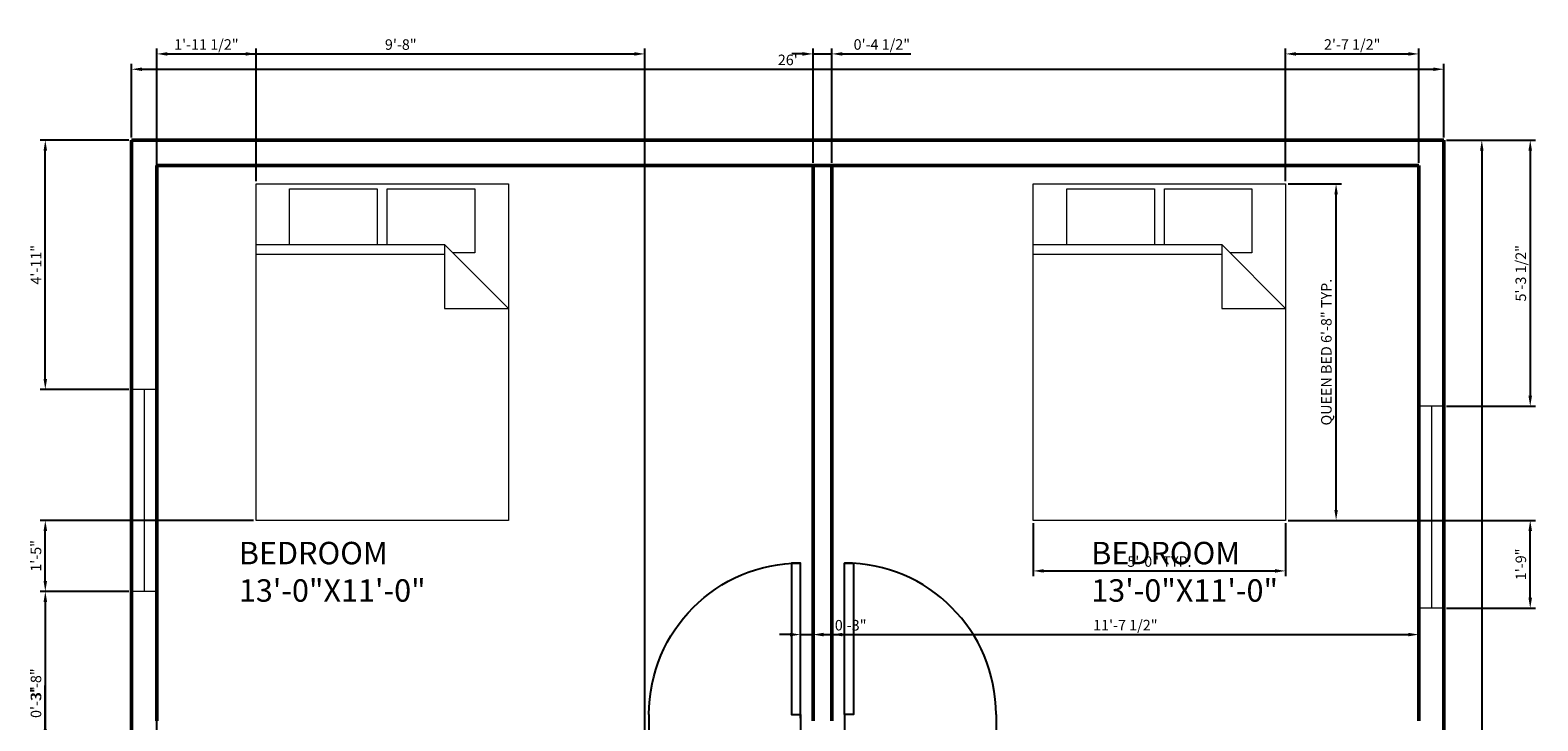
# Model space of a CAD drawing. Units: inches. Extents: x 158445 to 158806, y 254100 to 254533.
# Tile 3 of 3: x 158447 to 158806, y 254369 to 254533. Entities that reach past the tile are written whole.
import ezdxf

# ---------------------------------------------------------------- set-up
doc = ezdxf.new("R2010")
doc.units = ezdxf.units.IN
for name, color, linetype, lineweight in [('A-ANNO-DIMS', 2, 'Continuous', 18), ('A-AREA-IDEN', 7, 'Continuous', 25), ('A-DOOR', 3, 'Continuous', 25), ('A-FURN', 8, 'Continuous', 18), ('A-GLAZ', 4, 'Continuous', 18), ('A-WALL', 7, 'Continuous', 50)]:
    doc.layers.add(name, color=color, linetype=linetype, lineweight=lineweight)
doc.styles.get("Standard").update_dxf_attribs({"font": 'arial.ttf'})
doc.dimstyles.new('ISO-25', dxfattribs={"dimtxt": 2.5, "dimasz": 2.5, "dimexe": 1.25, "dimexo": 0.625, "dimtad": 1, "dimlunit": 4, "dimtxsty": 'Standard', "dimcen": 2.5, "dimadec": 0, "dimazin": 0, "dimtfac": 1, "dimtmove": 0, "dimatfit": 3, "dimfxl": 1, "dimarcsym": 0})

# ---------------------------------------------------------------- blocks, each defined once
blk = doc.blocks.new('*U2')
for p, q in [((0, 0), (0, -5)), ((30, 0), (30, -5))]:
    blk.add_line(p, q)
blk.add_lwpolyline([(0, 0), (0, 30), (1.75, 30), (1.75, 0)], close=True)
blk.add_arc((0, 0), 30, 0, 90)
blk = doc.blocks.new('Bed - Queen')
for p, q in [((0, -80.00003), (0, 0)), ((0, 0), (59.99999, 0)), ((59.99999, 0), (59.99999, -80.00003)), ((7.99999, -1.2), (28.79998, -1.2)), ((7.99999, -14.4), (7.99999, -1.2)), ((28.79998, -1.2), (28.79998, -14.4)), ((31.19999, -1.2), (51.99999, -1.2)), ((31.19999, -14.4), (31.19999, -1.2)), ((51.99999, -1.2), (51.99999, -16.4)), ((0, -14.4), (44.8, -14.4)), ((44.8, -16.8), (0, -16.8)), ((59.99999, -29.6), (44.8, -14.4)), ((44.8, -14.4), (44.8, -29.6)), ((51.99999, -16.4), (46.79936, -16.4)), ((44.8, -29.6), (59.99999, -29.6)), ((59.99999, -80.00003), (0, -80.00003))]:
    blk.add_line(p, q)
blk = doc.blocks.new('*D6')
at = {"layer": 'A-ANNO-DIMS', "color": 0, "lineweight": -2, "transparency": 16777216}
for p, q in [((158471.38, 254507.35), (158471.38, 254524.83)), ((158473.88, 254523.58), (158780.88, 254523.58)), ((158783.38, 254507.35), (158783.38, 254524.83))]:
    blk.add_line(p, q, dxfattribs=at)
at = {"layer": 'A-ANNO-DIMS', "color": 0, "transparency": 16777216}
for points in [[(158473.88, 254523.99), (158473.88, 254523.16), (158471.38, 254523.58)], [(158780.88, 254523.99), (158780.88, 254523.16), (158783.38, 254523.58)]]:
    blk.add_solid(points, dxfattribs=at)
at = {"layer": 'Defpoints', "color": 0, "transparency": 16777216}
for p in [(158783.38, 254523.58), (158471.38, 254506.72), (158783.38, 254506.72)]:
    blk.add_point(p, dxfattribs=at)
at = {"layer": 'A-ANNO-DIMS', "color": 0, "transparency": 16777216, "insert": (158627.38, 254525.48), "char_height": 2.5, "attachment_point": 5}
blk.add_mtext("26'", dxfattribs=at)
blk = doc.blocks.new('*D7')
at = {"layer": 'A-ANNO-DIMS', "color": 0, "lineweight": -2, "transparency": 16777216}
for p, q in [((158784.01, 254506.72), (158793.62, 254506.72)), ((158792.37, 254504.22), (158792.37, 254125.22)), ((158784.01, 254122.72), (158793.62, 254122.72))]:
    blk.add_line(p, q, dxfattribs=at)
at = {"layer": 'A-ANNO-DIMS', "color": 0, "transparency": 16777216}
for points in [[(158791.95, 254504.22), (158792.78, 254504.22), (158792.37, 254506.72)], [(158791.95, 254125.22), (158792.78, 254125.22), (158792.37, 254122.72)]]:
    blk.add_solid(points, dxfattribs=at)
at = {"layer": 'Defpoints', "color": 0, "transparency": 16777216}
for p in [(158783.38, 254506.72), (158783.38, 254122.72), (158792.37, 254122.72)]:
    blk.add_point(p, dxfattribs=at)
at = {"layer": 'A-ANNO-DIMS', "color": 0, "transparency": 16777216, "insert": (158790.47, 254314.72), "char_height": 2.5, "attachment_point": 5, "rotation": 90}
blk.add_mtext("32'", dxfattribs=at)
blk = doc.blocks.new('WIN-48IN')
for p, q in [((0, 6), (0, 0)), ((48, 6), (48, 0)), ((0, 3), (48, 3))]:
    blk.add_line(p, q)
blk = doc.blocks.new('*D10')
at = {"layer": 'A-ANNO-DIMS', "color": 0, "lineweight": -2, "transparency": 16777216}
for p, q in [((158746.36, 254496.35), (158758.98, 254496.35)), ((158757.73, 254418.85), (158757.73, 254493.85)), ((158746.36, 254416.35), (158758.98, 254416.35))]:
    blk.add_line(p, q, dxfattribs=at)
at = {"layer": 'A-ANNO-DIMS', "color": 0, "transparency": 16777216}
for points in [[(158757.32, 254493.85), (158758.15, 254493.85), (158757.73, 254496.35)], [(158757.32, 254418.85), (158758.15, 254418.85), (158757.73, 254416.35)]]:
    blk.add_solid(points, dxfattribs=at)
at = {"layer": 'Defpoints', "color": 0, "transparency": 16777216}
for p in [(158745.73, 254496.35), (158757.73, 254496.35), (158745.73, 254416.35)]:
    blk.add_point(p, dxfattribs=at)
at = {"layer": 'A-ANNO-DIMS', "color": 0, "transparency": 16777216, "insert": (158755.74, 254456.35), "char_height": 2.5, "attachment_point": 5, "rotation": 90}
blk.add_mtext('QUEEN BED 6\'-8" TYP.', dxfattribs=at)
blk = doc.blocks.new('*D11')
at = {"layer": 'A-ANNO-DIMS', "color": 0, "lineweight": -2, "transparency": 16777216}
for p, q in [((158685.73, 254415.73), (158685.73, 254403.1)), ((158745.73, 254415.73), (158745.73, 254403.1)), ((158688.23, 254404.35), (158743.23, 254404.35))]:
    blk.add_line(p, q, dxfattribs=at)
at = {"layer": 'A-ANNO-DIMS', "color": 0, "transparency": 16777216}
for points in [[(158688.23, 254404.77), (158688.23, 254403.94), (158685.73, 254404.35)], [(158743.23, 254404.77), (158743.23, 254403.94), (158745.73, 254404.35)]]:
    blk.add_solid(points, dxfattribs=at)
at = {"layer": 'Defpoints', "color": 0, "transparency": 16777216}
for p in [(158685.73, 254416.35), (158745.73, 254416.35), (158745.73, 254404.35)]:
    blk.add_point(p, dxfattribs=at)
at = {"layer": 'A-ANNO-DIMS', "color": 0, "transparency": 16777216, "insert": (158715.73, 254406.25), "char_height": 2.5, "attachment_point": 5}
blk.add_mtext('5\'-0" TYP.', dxfattribs=at)
blk = doc.blocks.new('*D18')
at = {"layer": 'A-ANNO-DIMS', "color": 0, "lineweight": -2, "transparency": 16777216}
for p, q in [((158470.76, 254506.72), (158449.63, 254506.72)), ((158450.88, 254449.98), (158450.88, 254504.22)), ((158470.76, 254447.48), (158449.63, 254447.48))]:
    blk.add_line(p, q, dxfattribs=at)
at = {"layer": 'A-ANNO-DIMS', "color": 0, "transparency": 16777216}
for points in [[(158450.46, 254504.22), (158451.3, 254504.22), (158450.88, 254506.72)], [(158450.46, 254449.98), (158451.3, 254449.98), (158450.88, 254447.48)]]:
    blk.add_solid(points, dxfattribs=at)
at = {"layer": 'Defpoints', "color": 0, "transparency": 16777216}
for p in [(158450.88, 254506.72), (158471.38, 254506.72), (158471.38, 254447.48)]:
    blk.add_point(p, dxfattribs=at)
at = {"layer": 'A-ANNO-DIMS', "color": 0, "transparency": 16777216, "insert": (158449, 254477.1), "char_height": 2.5, "attachment_point": 5, "rotation": 90}
blk.add_mtext('4\'-11"', dxfattribs=at)
blk = doc.blocks.new('*D19')
at = {"layer": 'A-ANNO-DIMS', "color": 0, "lineweight": -2, "transparency": 16777216}
for p, q in [((158470.76, 254399.48), (158449.63, 254399.48)), ((158450.88, 254396.98), (158450.88, 254357.89)), ((158470.76, 254355.39), (158449.63, 254355.39))]:
    blk.add_line(p, q, dxfattribs=at)
at = {"layer": 'A-ANNO-DIMS', "color": 0, "transparency": 16777216}
for points in [[(158450.46, 254396.98), (158451.3, 254396.98), (158450.88, 254399.48)], [(158450.46, 254357.89), (158451.3, 254357.89), (158450.88, 254355.39)]]:
    blk.add_solid(points, dxfattribs=at)
at = {"layer": 'Defpoints', "color": 0, "transparency": 16777216}
for p in [(158471.38, 254399.48), (158450.88, 254355.39), (158471.38, 254355.39)]:
    blk.add_point(p, dxfattribs=at)
at = {"layer": 'A-ANNO-DIMS', "color": 0, "transparency": 16777216, "insert": (158448.98, 254377.43), "char_height": 2.5, "attachment_point": 5, "rotation": 90}
blk.add_mtext('3\'-8"', dxfattribs=at)
blk = doc.blocks.new('*D21')
at = {"layer": 'A-ANNO-DIMS', "color": 0, "lineweight": -2, "transparency": 16777216}
for p, q in [((158784.01, 254506.72), (158805.13, 254506.72)), ((158803.88, 254504.22), (158803.88, 254445.97)), ((158784.01, 254443.47), (158805.13, 254443.47))]:
    blk.add_line(p, q, dxfattribs=at)
at = {"layer": 'A-ANNO-DIMS', "color": 0, "transparency": 16777216}
for points in [[(158803.46, 254504.22), (158804.3, 254504.22), (158803.88, 254506.72)], [(158803.46, 254445.97), (158804.3, 254445.97), (158803.88, 254443.47)]]:
    blk.add_solid(points, dxfattribs=at)
at = {"layer": 'Defpoints', "color": 0, "transparency": 16777216}
for p in [(158783.38, 254506.72), (158783.38, 254443.47), (158803.88, 254443.47)]:
    blk.add_point(p, dxfattribs=at)
at = {"layer": 'A-ANNO-DIMS', "color": 0, "transparency": 16777216, "insert": (158801.96, 254475.09), "char_height": 2.5, "attachment_point": 5, "rotation": 90}
blk.add_mtext('5\'-3 1/2"', dxfattribs=at)
blk = doc.blocks.new('*D27')
at = {"layer": 'A-ANNO-DIMS', "color": 0, "lineweight": -2, "transparency": 16777216}
for p, q in [((158637.88, 254369.35), (158637.88, 254390.47)), ((158640.38, 254389.22), (158774.88, 254389.22)), ((158777.38, 254369.35), (158777.38, 254390.47))]:
    blk.add_line(p, q, dxfattribs=at)
at = {"layer": 'A-ANNO-DIMS', "color": 0, "transparency": 16777216}
for points in [[(158640.38, 254389.64), (158640.38, 254388.8), (158637.88, 254389.22)], [(158774.88, 254389.64), (158774.88, 254388.8), (158777.38, 254389.22)]]:
    blk.add_solid(points, dxfattribs=at)
at = {"layer": 'Defpoints', "color": 0, "transparency": 16777216}
for p in [(158777.38, 254389.22), (158637.88, 254368.72), (158777.38, 254368.72)]:
    blk.add_point(p, dxfattribs=at)
at = {"layer": 'A-ANNO-DIMS', "color": 0, "transparency": 16777216, "insert": (158707.63, 254391.14), "char_height": 2.5, "attachment_point": 5}
blk.add_mtext('11\'-7 1/2"', dxfattribs=at)
blk = doc.blocks.new('*D30')
at = {"layer": 'A-ANNO-DIMS', "color": 0, "lineweight": -2, "transparency": 16777216}
for p, q in [((158477.38, 254364.85), (158477.38, 254528.47)), ((158479.88, 254527.22), (158590.88, 254527.22)), ((158593.38, 254364.85), (158593.38, 254528.47))]:
    blk.add_line(p, q, dxfattribs=at)
at = {"layer": 'A-ANNO-DIMS', "color": 0, "transparency": 16777216}
for points in [[(158479.88, 254527.64), (158479.88, 254526.8), (158477.38, 254527.22)], [(158590.88, 254527.64), (158590.88, 254526.8), (158593.38, 254527.22)]]:
    blk.add_solid(points, dxfattribs=at)
at = {"layer": 'Defpoints', "color": 0, "transparency": 16777216}
for p in [(158593.38, 254527.22), (158477.38, 254364.22), (158593.38, 254364.22)]:
    blk.add_point(p, dxfattribs=at)
at = {"layer": 'A-ANNO-DIMS', "color": 0, "transparency": 16777216, "insert": (158535.38, 254529.12), "char_height": 2.5, "attachment_point": 5}
blk.add_mtext('9\'-8"', dxfattribs=at)
blk = doc.blocks.new('*D37')
at = {"layer": 'A-ANNO-DIMS', "color": 0, "lineweight": -2, "transparency": 16777216}
for p, q in [((158630.88, 254527.22), (158628.38, 254527.22)), ((158633.38, 254501.35), (158633.38, 254528.47)), ((158633.38, 254527.22), (158637.88, 254527.22)), ((158637.88, 254501.35), (158637.88, 254528.47)), ((158640.38, 254527.22), (158656.6, 254527.22))]:
    blk.add_line(p, q, dxfattribs=at)
at = {"layer": 'A-ANNO-DIMS', "color": 0, "transparency": 16777216}
for points in [[(158630.88, 254527.64), (158630.88, 254526.8), (158633.38, 254527.22)], [(158640.38, 254527.64), (158640.38, 254526.8), (158637.88, 254527.22)]]:
    blk.add_solid(points, dxfattribs=at)
at = {"layer": 'Defpoints', "color": 0, "transparency": 16777216}
for p in [(158637.88, 254527.22), (158633.38, 254500.72), (158637.88, 254500.72)]:
    blk.add_point(p, dxfattribs=at)
at = {"layer": 'A-ANNO-DIMS', "color": 0, "transparency": 16777216, "insert": (158649.74, 254529.14), "char_height": 2.5, "attachment_point": 5}
blk.add_mtext('0\'-4 1/2"', dxfattribs=at)
blk = doc.blocks.new('*D44')
at = {"layer": 'A-ANNO-DIMS', "color": 0, "lineweight": -2, "transparency": 16777216}
for p, q in [((158627.88, 254389.22), (158625.38, 254389.22)), ((158630.38, 254369.35), (158630.38, 254390.47)), ((158630.38, 254389.22), (158633.38, 254389.22)), ((158633.38, 254369.35), (158633.38, 254390.47)), ((158635.88, 254389.22), (158646.28, 254389.22))]:
    blk.add_line(p, q, dxfattribs=at)
at = {"layer": 'A-ANNO-DIMS', "color": 0, "transparency": 16777216}
for points in [[(158627.88, 254389.64), (158627.88, 254388.8), (158630.38, 254389.22)], [(158635.88, 254389.64), (158635.88, 254388.8), (158633.38, 254389.22)]]:
    blk.add_solid(points, dxfattribs=at)
at = {"layer": 'Defpoints', "color": 0, "transparency": 16777216}
for p in [(158633.38, 254389.22), (158630.38, 254368.72), (158633.38, 254368.72)]:
    blk.add_point(p, dxfattribs=at)
at = {"layer": 'A-ANNO-DIMS', "color": 0, "transparency": 16777216, "insert": (158642.33, 254391.12), "char_height": 2.5, "attachment_point": 5}
blk.add_mtext('0\'-3"', dxfattribs=at)
blk = doc.blocks.new('*D45')
at = {"layer": 'A-ANNO-DIMS', "color": 0, "lineweight": -2, "transparency": 16777216}
for p, q in [((158477.38, 254501.35), (158477.38, 254528.47)), ((158479.88, 254527.22), (158498.47, 254527.22)), ((158500.97, 254496.98), (158500.97, 254528.47))]:
    blk.add_line(p, q, dxfattribs=at)
at = {"layer": 'A-ANNO-DIMS', "color": 0, "transparency": 16777216}
for points in [[(158479.88, 254527.64), (158479.88, 254526.8), (158477.38, 254527.22)], [(158498.47, 254527.64), (158498.47, 254526.8), (158500.97, 254527.22)]]:
    blk.add_solid(points, dxfattribs=at)
at = {"layer": 'Defpoints', "color": 0, "transparency": 16777216}
for p in [(158500.97, 254527.22), (158477.38, 254500.72), (158500.97, 254496.35)]:
    blk.add_point(p, dxfattribs=at)
at = {"layer": 'A-ANNO-DIMS', "color": 0, "transparency": 16777216, "insert": (158489.17, 254529.14), "char_height": 2.5, "attachment_point": 5}
blk.add_mtext('1\'-11 1/2"', dxfattribs=at)
blk = doc.blocks.new('*D46')
at = {"layer": 'A-ANNO-DIMS', "color": 0, "lineweight": -2, "transparency": 16777216}
for p, q in [((158745.73, 254496.98), (158745.73, 254528.47)), ((158748.23, 254527.22), (158774.88, 254527.22)), ((158777.38, 254501.35), (158777.38, 254528.47))]:
    blk.add_line(p, q, dxfattribs=at)
at = {"layer": 'A-ANNO-DIMS', "color": 0, "transparency": 16777216}
for points in [[(158748.23, 254527.64), (158748.23, 254526.8), (158745.73, 254527.22)], [(158774.88, 254527.64), (158774.88, 254526.8), (158777.38, 254527.22)]]:
    blk.add_solid(points, dxfattribs=at)
at = {"layer": 'Defpoints', "color": 0, "transparency": 16777216}
for p in [(158777.38, 254527.22), (158777.38, 254500.72), (158745.73, 254496.35)]:
    blk.add_point(p, dxfattribs=at)
at = {"layer": 'A-ANNO-DIMS', "color": 0, "transparency": 16777216, "insert": (158761.56, 254529.14), "char_height": 2.5, "attachment_point": 5}
blk.add_mtext('2\'-7 1/2"', dxfattribs=at)
blk = doc.blocks.new('*D47')
at = {"layer": 'A-ANNO-DIMS', "color": 0, "lineweight": -2, "transparency": 16777216}
for p, q in [((158500.34, 254416.35), (158449.63, 254416.35)), ((158450.88, 254401.98), (158450.88, 254413.85)), ((158470.76, 254399.48), (158449.63, 254399.48))]:
    blk.add_line(p, q, dxfattribs=at)
at = {"layer": 'A-ANNO-DIMS', "color": 0, "transparency": 16777216}
for points in [[(158450.46, 254413.85), (158451.3, 254413.85), (158450.88, 254416.35)], [(158450.46, 254401.98), (158451.3, 254401.98), (158450.88, 254399.48)]]:
    blk.add_solid(points, dxfattribs=at)
at = {"layer": 'Defpoints', "color": 0, "transparency": 16777216}
for p in [(158450.88, 254416.35), (158500.97, 254416.35), (158471.38, 254399.48)]:
    blk.add_point(p, dxfattribs=at)
at = {"layer": 'A-ANNO-DIMS', "color": 0, "transparency": 16777216, "insert": (158448.98, 254407.92), "char_height": 2.5, "attachment_point": 5, "rotation": 90}
blk.add_mtext('1\'-5"', dxfattribs=at)
blk = doc.blocks.new('*D48')
at = {"layer": 'A-ANNO-DIMS', "color": 0, "lineweight": -2, "transparency": 16777216}
for p, q in [((158746.36, 254416.35), (158805.13, 254416.35)), ((158803.88, 254397.97), (158803.88, 254413.85)), ((158784.01, 254395.47), (158805.13, 254395.47))]:
    blk.add_line(p, q, dxfattribs=at)
at = {"layer": 'A-ANNO-DIMS', "color": 0, "transparency": 16777216}
for points in [[(158803.46, 254413.85), (158804.3, 254413.85), (158803.88, 254416.35)], [(158803.46, 254397.97), (158804.3, 254397.97), (158803.88, 254395.47)]]:
    blk.add_solid(points, dxfattribs=at)
at = {"layer": 'Defpoints', "color": 0, "transparency": 16777216}
for p in [(158745.73, 254416.35), (158803.88, 254416.35), (158783.38, 254395.47)]:
    blk.add_point(p, dxfattribs=at)
at = {"layer": 'A-ANNO-DIMS', "color": 0, "transparency": 16777216, "insert": (158801.98, 254405.91), "char_height": 2.5, "attachment_point": 5, "rotation": 90}
blk.add_mtext('1\'-9"', dxfattribs=at)
blk = doc.blocks.new('*D53')
at = {"layer": 'A-ANNO-DIMS', "color": 0, "lineweight": -2, "transparency": 16777216}
for p, q in [((158450.88, 254366.72), (158450.88, 254377.12)), ((158728.76, 254364.22), (158449.63, 254364.22)), ((158450.88, 254361.22), (158450.88, 254364.22)), ((158728.76, 254361.22), (158449.63, 254361.22)), ((158450.88, 254358.72), (158450.88, 254356.22))]:
    blk.add_line(p, q, dxfattribs=at)
at = {"layer": 'A-ANNO-DIMS', "color": 0, "transparency": 16777216}
for points in [[(158450.46, 254366.72), (158451.3, 254366.72), (158450.88, 254364.22)], [(158450.46, 254358.72), (158451.3, 254358.72), (158450.88, 254361.22)]]:
    blk.add_solid(points, dxfattribs=at)
at = {"layer": 'Defpoints', "color": 0, "transparency": 16777216}
for p in [(158450.88, 254364.22), (158729.38, 254364.22), (158729.38, 254361.22)]:
    blk.add_point(p, dxfattribs=at)
at = {"layer": 'A-ANNO-DIMS', "color": 0, "transparency": 16777216, "insert": (158448.98, 254373.17), "char_height": 2.5, "attachment_point": 5, "rotation": 90}
blk.add_mtext('0\'-3"', dxfattribs=at)

msp = doc.modelspace()

# ---------------------------------------------------------------- linework, layer by layer
at = {"layer": 'A-WALL'}
for p, q in [((158783.381, 254506.721), (158471.381, 254506.721)), ((158471.381, 254506.721), (158471.381, 254122.721)), ((158783.381, 254122.721), (158783.381, 254506.721)), ((158777.381, 254500.721), (158477.381, 254500.721)), ((158477.381, 254500.721), (158477.381, 254368.721)), ((158633.381, 254500.721), (158633.381, 254368.721)), ((158637.881, 254500.721), (158637.881, 254368.721)), ((158777.381, 254368.721), (158777.381, 254500.721))]:
    msp.add_line(p, q, dxfattribs=at)

# ---------------------------------------------------------------- block references
at = {"layer": 'A-DOOR', "yscale": 1.199999999999999, "zscale": 1.199999999999999}
for p, xscale in [((158630.381, 254370.221), -1.199999999999999), ((158640.881, 254370.221), 1.199999999999999)]:
    msp.add_blockref('*U2', p, dxfattribs=dict(at, xscale=xscale))
at = {"layer": 'A-FURN'}
for p in [(158500.966, 254496.353), (158685.734, 254496.353)]:
    msp.add_blockref('Bed - Queen', p, dxfattribs=at)
at = {"layer": 'A-GLAZ'}
for p, rotation in [((158471.381, 254447.482), 269.9999999998033), ((158777.381, 254443.466), 269.9999999999487)]:
    msp.add_blockref('WIN-48IN', p, dxfattribs=dict(at, rotation=rotation))

# ---------------------------------------------------------------- texts
at = {"layer": 'A-AREA-IDEN', "char_height": 5.335, "attachment_point": 1}
for insert in [(158496.887, 254411.258), (158699.519, 254411.258)]:
    msp.add_mtext_dynamic_manual_height_columns('BEDROOM\\P13\'-0"X11\'-0"', width=5.37287, gutter_width=26.675, heights=[0], dxfattribs=dict(at, insert=insert))

# ---------------------------------------------------------------- dimensions: what is measured, and where the dimension line sits
at = {"layer": 'A-ANNO-DIMS'}
for base, p1, p2, override, picture, middle in [((158500.966, 254527.221), (158477.381, 254500.721), (158500.966, 254496.353), {"dimdec": 1, "dimlfac": 1, "dimrnd": 0, "dimzin": 1, "dimdsep": 46, "dimlunit": 4, "dimfrac": 2}, '*D45', (158489.174, 254529.139)), ((158637.881, 254527.221), (158633.381, 254500.721), (158637.881, 254500.721), {"dimdec": 1, "dimlfac": 1, "dimrnd": 0, "dimzin": 1, "dimdsep": 46, "dimlunit": 4, "dimfrac": 2}, '*D37', (158649.742, 254529.139)), ((158777.381, 254527.221), (158745.734, 254496.353), (158777.381, 254500.721), {"dimdec": 1, "dimlfac": 1, "dimrnd": 0, "dimzin": 1, "dimdsep": 46, "dimlunit": 4, "dimfrac": 2}, '*D46', (158761.558, 254529.139)), ((158593.381, 254527.221), (158477.381, 254364.221), (158593.381, 254364.221), {"dimdec": 1, "dimlfac": 1, "dimrnd": 0, "dimzin": 1, "dimdsep": 46, "dimlunit": 4, "dimfrac": 2}, '*D30', (158535.381, 254529.122)), ((158783.381, 254523.577), (158471.381, 254506.721), (158783.381, 254506.721), {"dimclrd": 0, "dimclre": 0, "dimclrt": 0}, '*D6', (158627.381, 254525.478)), ((158777.381, 254389.221), (158637.881, 254368.721), (158777.381, 254368.721), {"dimdec": 1, "dimlfac": 1, "dimrnd": 0, "dimzin": 1, "dimdsep": 46, "dimlunit": 4, "dimfrac": 2}, '*D27', (158707.631, 254391.139))]:
    dim = msp.add_linear_dim(base=base, p1=p1, p2=p2, dimstyle='ISO-25', override=override, dxfattribs=at)
    dim.commit()
    dim.dimension.update_dxf_attribs({"geometry": picture, "text_midpoint": middle})
for base, p1, p2, angle, override, picture, middle in [((158450.881, 254506.721), (158471.381, 254447.482), (158471.381, 254506.721), 90, {"dimdec": 1, "dimlfac": 1, "dimrnd": 0, "dimzin": 1, "dimdsep": 46, "dimlunit": 4, "dimfrac": 2}, '*D18', (158449.001, 254477.102)), ((158792.368, 254122.721), (158783.381, 254506.721), (158783.381, 254122.721), 90, {"dimclrd": 0, "dimclre": 0, "dimclrt": 0}, '*D7', (158790.465, 254314.721)), ((158803.881, 254443.466), (158783.381, 254506.721), (158783.381, 254443.466), 90, {"dimdec": 1, "dimlfac": 1, "dimrnd": 0, "dimzin": 1, "dimdsep": 46, "dimlunit": 4, "dimfrac": 2}, '*D21', (158801.963, 254475.093)), ((158450.881, 254416.353), (158471.381, 254399.482), (158500.966, 254416.353), 90, {"dimdec": 1, "dimlfac": 1, "dimrnd": 0, "dimzin": 1, "dimdsep": 46, "dimlunit": 4, "dimfrac": 2}, '*D47', (158448.98, 254407.917)), ((158803.881, 254416.353), (158783.381, 254395.466), (158745.734, 254416.353), 90, {"dimdec": 1, "dimlfac": 1, "dimrnd": 0, "dimzin": 1, "dimdsep": 46, "dimlunit": 4, "dimfrac": 2}, '*D48', (158801.98, 254405.909)), ((158450.881, 254355.388), (158471.381, 254399.482), (158471.381, 254355.388), 90, {"dimdec": 1, "dimlfac": 1, "dimrnd": 0, "dimzin": 1, "dimdsep": 46, "dimlunit": 4, "dimfrac": 2}, '*D19', (158448.979, 254377.435)), ((158633.381, 254389.221), (158630.381, 254368.721), (158633.381, 254368.721), 360, {"dimdec": 1, "dimlfac": 1, "dimrnd": 0, "dimzin": 1, "dimdsep": 46, "dimlunit": 4, "dimfrac": 2}, '*D44', (158642.329, 254391.123)), ((158450.881, 254364.221), (158729.381, 254361.221), (158729.381, 254364.221), 90, {"dimdec": 1, "dimlfac": 1, "dimrnd": 0, "dimzin": 1, "dimdsep": 46, "dimlunit": 4, "dimfrac": 2}, '*D53', (158448.979, 254373.169))]:
    dim = msp.add_linear_dim(base=base, p1=p1, p2=p2, angle=angle, dimstyle='ISO-25', override=override, dxfattribs=at)
    dim.commit()
    dim.dimension.update_dxf_attribs({"geometry": picture, "text_midpoint": middle})
dim = msp.add_linear_dim(base=(158757.734, 254496.353), p1=(158745.734, 254416.353), p2=(158745.734, 254496.353), angle=90, text='QUEEN BED <> TYP.', dimstyle='ISO-25', override={"dimdec": 1, "dimlfac": 1, "dimrnd": 0, "dimzin": 1, "dimdsep": 46, "dimlunit": 4, "dimfrac": 2}, dxfattribs=at)
dim.commit()
dim.dimension.update_dxf_attribs({"geometry": '*D10', "text_midpoint": (158755.74, 254456.353)})
dim = msp.add_linear_dim(base=(158745.734, 254404.353), p1=(158685.734, 254416.353), p2=(158745.734, 254416.353), text='<> TYP.', dimstyle='ISO-25', override={"dimdec": 1, "dimlfac": 1, "dimrnd": 0, "dimzin": 1, "dimdsep": 46, "dimlunit": 4, "dimfrac": 2}, dxfattribs=at)
dim.commit()
dim.dimension.update_dxf_attribs({"geometry": '*D11', "text_midpoint": (158715.734, 254406.254)})

doc.saveas('drawing.dxf')
